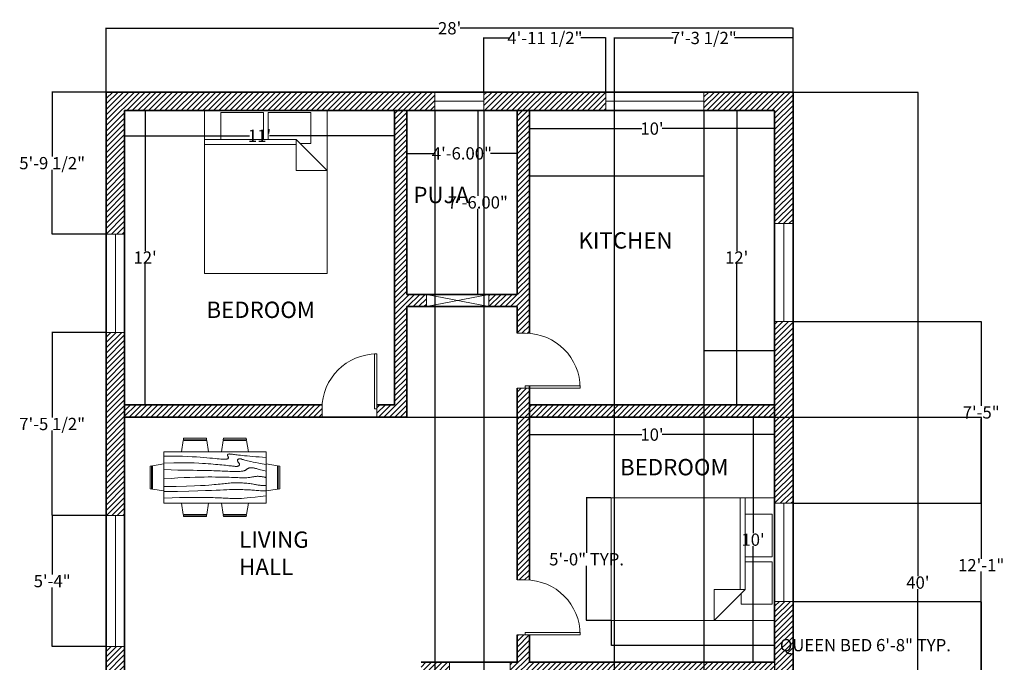
# Model space of a CAD drawing. Units: inches. Extents: x -20 to 887, y -143 to 410.
# Tile 5 of 5: x 401 to 883, y 96 to 410. Entities that reach past the tile are written whole.
import ezdxf

# ---------------------------------------------------------------- set-up
doc = ezdxf.new("R2010")
doc.units = ezdxf.units.IN
doc.header["$MEASUREMENT"] = 0
for name, color, linetype, lineweight in [('A-ANNO-DIMS', 2, 'Continuous', 18), ('A-AREA-IDEN', 7, 'Continuous', 25), ('A-DOOR', 3, 'Continuous', 18), ('A-FLOR-CASE', 9, 'Continuous', 25), ('A-FURN', 8, 'Continuous', 18), ('A-GLAZ', 4, 'Continuous', 18), ('A-WALL', 7, 'Continuous', 35), ('A-WALL-PATT', 8, 'Continuous', 13)]:
    doc.layers.add(name, color=color, linetype=linetype, lineweight=lineweight)
doc.styles.get("Standard").update_dxf_attribs({"font": 'arial.ttf'})
doc.dimstyles.get("Standard").update_dxf_attribs({"dimtxt": 6, "dimasz": 0.18, "dimexe": 0.18, "dimexo": 0.0625, "dimgap": 0.09, "dimtad": 0, "dimtih": 1, "dimtoh": 1, "dimzin": 0, "dimdsep": 46, "dimlunit": 3, "dimtxsty": 'Standard', "dimcen": 0.09, "dimadec": 0, "dimazin": 0, "dimtfac": 1, "dimtofl": 0, "dimtmove": 0, "dimatfit": 3, "dimfxl": 1, "dimtolj": 1, "dimtzin": 0, "dimarcsym": 0})

# ---------------------------------------------------------------- blocks, each defined once
blk = doc.blocks.new('Bed - Queen')
for p, q in [((0, -80.00003), (0, 0)), ((0, 0), (59.99999, 0)), ((59.99999, 0), (59.99999, -80.00003)), ((7.99999, -1.2), (28.79998, -1.2)), ((7.99999, -14.4), (7.99999, -1.2)), ((28.79998, -1.2), (28.79998, -14.4)), ((31.19999, -1.2), (51.99999, -1.2)), ((31.19999, -14.4), (31.19999, -1.2)), ((51.99999, -1.2), (51.99999, -16.4)), ((0, -14.4), (44.8, -14.4)), ((59.99999, -29.6), (44.8, -14.4)), ((44.8, -14.4), (44.8, -29.6)), ((44.8, -16.8), (0, -16.8)), ((51.99999, -16.4), (46.79936, -16.4)), ((44.8, -29.6), (59.99999, -29.6)), ((59.99999, -80.00003), (0, -80.00003))]:
    blk.add_line(p, q)
blk = doc.blocks.new('*U2')
for p, q in [((0, 0), (0, -6)), ((40, 0), (40, -6))]:
    blk.add_line(p, q)
blk.add_lwpolyline([(0, 0), (0, 40), (1.75, 40), (1.75, 0)], close=True)
blk.add_arc((0, 0), 40, 0, 90)
blk = doc.blocks.new('Dining Set - 36 x 72 in.')
for p, q in [((-22.2343, 26.00059), (-23.4847, 17.99762)), ((-22.2304, 26), (-5.7608, 26)), ((-22, 27.5), (-22.1562, 26.50042)), ((-5.8416, 26.5), (-22.1534, 26.5)), ((-22, 27.5), (-6, 27.5)), ((-5.8437, 26.49966), (-6, 27.5)), ((-4.5152, 17.99762), (-5.7655, 25.99926)), ((5.7657, 26.00059), (4.5153, 17.99762)), ((5.7696, 26), (22.2392, 26)), ((6, 27.5), (5.8438, 26.50042)), ((22.1584, 26.5), (5.8466, 26.5)), ((6, 27.5), (22, 27.5)), ((22.1563, 26.49966), (22, 27.5)), ((23.4848, 17.99762), (22.2345, 25.99926)), ((36, 18), (-36, 18)), ((-36, 18), (-36, -18)), ((36, -18), (36, 18)), ((-45.5, 8), (-44.5004, 8.15617)), ((-45.5, 8), (-45.5, -8)), ((-44.5, -8.15843), (-44.5, 8.15338)), ((-44.0006, 8.23428), (-35.9976, 9.48474)), ((-44, 8.23041), (-44, -8.23915)), ((44.0006, 8.23428), (35.9976, 9.48474)), ((44, 8.23041), (44, -8.23915)), ((44.5, -8.15843), (44.5, 8.15338)), ((45.5, 8), (44.5005, 8.15617)), ((45.5, 8), (45.5, -8)), ((-44.4997, -8.15631), (-45.5, -8)), ((-35.9976, -9.48476), (-43.9993, -8.2345)), ((35.9976, -9.48476), (43.9993, -8.2345)), ((44.4997, -8.15631), (45.5, -8)), ((-36, -18), (36, -18)), ((-22.2343, -26.0006), (-23.4847, -17.99762)), ((-4.5152, -17.99762), (-5.7655, -25.99928)), ((5.7657, -26.0006), (4.5153, -17.99762)), ((23.4848, -17.99762), (22.2345, -25.99928)), ((-22.2304, -26), (-5.7608, -26)), ((-22, -27.5), (-22.1562, -26.50044)), ((-5.8416, -26.5), (-22.1534, -26.5)), ((-22, -27.5), (-6, -27.5)), ((-5.8437, -26.49967), (-6, -27.5)), ((5.7696, -26), (22.2392, -26)), ((6, -27.5), (5.8438, -26.50044)), ((22.1584, -26.5), (5.8466, -26.5)), ((6, -27.5), (22, -27.5)), ((22.1563, -26.49967), (22, -27.5))]:
    blk.add_line(p, q)
for points in [[(-36, 15), (-31.1772, 14.97754), (-26.8079, 14.91406), (-22.8538, 14.81543), (-19.276, 14.6875), (-16.0362, 14.53613), (-13.0957, 14.36718), (-10.4159, 14.18652), (-7.9583, 14), (-5.6904, 13.81315), (-3.6035, 13.63021), (-1.6954, 13.45508), (0.0365, 13.29166), (1.5945, 13.14388), (2.9811, 13.01562), (4.1988, 12.9108), (5.25, 12.83333), (6.1393, 12.78613), (6.8802, 12.76823), (7.4883, 12.77767), (7.9792, 12.8125), (8.3685, 12.87077), (8.6719, 12.95052), (8.9049, 13.0498), (9.0833, 13.16666), (9.2205, 13.29899), (9.3216, 13.44401), (9.3895, 13.59879), (9.4271, 13.76041), (9.4373, 13.92594), (9.4232, 14.09245), (9.3875, 14.257), (9.3333, 14.41666), (9.2638, 14.56917), (9.1836, 14.71484), (9.0975, 14.85465), (9.0104, 14.98958), (8.9272, 15.1206), (8.8529, 15.2487), (8.7922, 15.37483), (8.75, 15.5), (8.7305, 15.62467), (8.7344, 15.74739), (8.7617, 15.86621), (8.8125, 15.97916), (8.8867, 16.08431), (8.9844, 16.17968), (9.1055, 16.26334), (9.25, 16.33333), (9.4189, 16.38802), (9.6172, 16.42708), (9.8506, 16.45052), (10.125, 16.45833), (10.4463, 16.45052), (10.8203, 16.42708), (11.2529, 16.38802), (11.75, 16.33333), (12.3184, 16.26318), (12.9694, 16.17838), (13.7151, 16.07991), (14.5677, 15.96875), (15.5395, 15.84586), (16.6426, 15.71224), (17.8893, 15.56884), (19.2917, 15.41666), (20.859, 15.25667), (22.5879, 15.08984), (24.4721, 14.91715), (26.5052, 14.73958), (28.6809, 14.5581), (30.9929, 14.3737), (33.4347, 14.18733), (36, 14)], [(-36, 10), (-28.9766, 10.14274), (-23.1725, 10.20442), (-18.4241, 10.19775), (-14.5677, 10.13541), (-11.4399, 10.03011), (-8.877, 9.89453), (-6.7154, 9.74137), (-4.7917, 9.58333), (-2.9698, 9.43082), (-1.2246, 9.28515), (0.4415, 9.14534), (2.026, 9.01041), (3.5266, 8.87939), (4.9408, 8.7513), (6.266, 8.62516), (7.5, 8.5), (8.6411, 8.37549), (9.6914, 8.2539), (10.6538, 8.13818), (11.5312, 8.03125), (12.3267, 7.93603), (13.043, 7.85547), (13.6831, 7.79248), (14.25, 7.75), (14.7471, 7.7303), (15.1797, 7.73307), (15.5537, 7.75732), (15.875, 7.80208), (16.1494, 7.86637), (16.3828, 7.94922), (16.5811, 8.04964), (16.75, 8.16666), (16.8944, 8.29915), (17.0143, 8.44531), (17.1089, 8.60319), (17.1771, 8.77083), (17.218, 8.94629), (17.2305, 9.1276), (17.2137, 9.31282), (17.1667, 9.5), (17.0895, 9.6875), (16.987, 9.875), (16.8649, 10.0625), (16.7292, 10.25), (16.5856, 10.4375), (16.4401, 10.625), (16.2985, 10.8125), (16.1667, 11), (16.05, 11.18733), (15.9518, 11.3737), (15.8752, 11.5581), (15.8229, 11.73958), (15.798, 11.91715), (15.8034, 12.08984), (15.842, 12.25667), (15.9167, 12.41666), (16.0295, 12.56836), (16.1784, 12.70833), (16.3605, 12.83268), (16.5729, 12.9375), (16.8127, 13.01888), (17.0768, 13.07291), (17.3625, 13.0957), (17.6667, 13.08333), (17.9894, 13.03312), (18.3418, 12.94726), (18.7382, 12.82918), (19.1927, 12.68229), (19.7195, 12.51001), (20.3327, 12.31575), (21.0465, 12.10294), (21.875, 11.875), (22.8357, 11.63354), (23.959, 11.37304), (25.2786, 11.08618), (26.8282, 10.76562), (28.6414, 10.40405), (30.752, 9.99414), (33.1936, 9.52856), (36, 9)], [(-36, 5.5), (-30.7157, 5.3348), (-26.069, 5.20963), (-21.9946, 5.11767), (-18.4271, 5.05208), (-15.3009, 5.00602), (-12.5508, 4.97265), (-10.1112, 4.94515), (-7.9167, 4.91666), (-5.909, 4.88167), (-4.0586, 4.83984), (-2.3429, 4.79215), (-0.7396, 4.73958), (0.7739, 4.6831), (2.22, 4.6237), (3.6213, 4.56233), (5, 4.5), (6.373, 4.43782), (7.7344, 4.3776), (9.0723, 4.32129), (10.375, 4.27083), (11.6309, 4.22819), (12.8281, 4.19531), (13.9551, 4.17415), (15, 4.16666), (15.954, 4.17448), (16.819, 4.19791), (17.6001, 4.23698), (18.3021, 4.29166), (18.9299, 4.36198), (19.4883, 4.44791), (19.9823, 4.54948), (20.4167, 4.66666), (20.7969, 4.79899), (21.1302, 4.94401), (21.4245, 5.09879), (21.6875, 5.26041), (21.9271, 5.42594), (22.1511, 5.59245), (22.3672, 5.757), (22.5834, 5.91666), (22.8065, 6.06868), (23.0404, 6.21093), (23.2879, 6.34147), (23.5521, 6.45833), (23.8358, 6.55957), (24.142, 6.64323), (24.4735, 6.70735), (24.8334, 6.75), (25.2235, 6.76969), (25.642, 6.76692), (26.0858, 6.74267), (26.5521, 6.69791), (27.0379, 6.63362), (27.5404, 6.55078), (28.0565, 6.45036), (28.5834, 6.33333), (29.1242, 6.19987), (29.7071, 6.04687), (30.3661, 5.87044), (31.1354, 5.66666), (32.0493, 5.43164), (33.142, 5.16146), (34.4475, 4.85221), (36, 4.5)], [(-36, -1), (-30.7915, -0.6591), (-26.0195, -0.38216), (-21.6519, -0.16284), (-17.6563, 0.00521), (-14.0005, 0.12833), (-10.6523, 0.21289), (-7.5796, 0.26522), (-4.75, 0.29166), (-2.134, 0.29793), (0.2878, 0.28711), (2.5317, 0.26163), (4.6146, 0.22396), (6.5529, 0.17651), (8.3633, 0.12174), (10.0623, 0.06209), (11.6667, 0), (13.1899, -0.06201), (14.6341, -0.1211), (15.9982, -0.17432), (17.2813, -0.21875), (18.4823, -0.25147), (19.6003, -0.26953), (20.6343, -0.27002), (21.5834, -0.25), (22.4481, -0.20768), (23.2357, -0.14584), (23.9549, -0.06836), (24.6146, 0.02083), (25.2235, 0.11784), (25.7904, 0.21875), (26.3241, 0.31966), (26.8334, 0.41666), (27.3265, 0.50618), (27.8099, 0.58593), (28.2894, 0.65397), (28.7709, 0.70833), (29.2601, 0.74707), (29.763, 0.76823), (30.2855, 0.76985), (30.8334, 0.75), (31.4088, 0.70784), (31.9994, 0.64713), (32.589, 0.57275), (33.1615, 0.48958), (33.7008, 0.4025), (34.1908, 0.3164), (34.6153, 0.23616), (34.9584, 0.16666), (35.2099, 0.11165), (35.3848, 0.07031), (35.504, 0.04069), (35.5886, 0.02083), (35.6594, 0.00879), (35.7377, 0.0026), (35.8442, 0.00032), (36, 0)], [(-36, -6.5), (-27.1843, -6.31267), (-20.084, -6.1263), (-14.469, -5.9419), (-10.1094, -5.76042), (-6.7752, -5.58285), (-4.2363, -5.41016), (-2.2629, -5.24333), (-0.625, -5.08334), (0.8708, -4.93099), (2.2715, -4.78646), (3.5872, -4.64974), (4.8281, -4.52084), (6.0046, -4.39974), (7.127, -4.28646), (8.2053, -4.18099), (9.25, -4.08334), (10.2705, -3.99382), (11.2734, -3.91407), (12.2647, -3.84603), (13.25, -3.79167), (14.2354, -3.75293), (15.2266, -3.73177), (16.2295, -3.73015), (17.25, -3.75), (18.2912, -3.79248), (19.3451, -3.85547), (20.4009, -3.93604), (21.4479, -4.03125), (22.4754, -4.13819), (23.4727, -4.25391), (24.4289, -4.37549), (25.3334, -4.5), (26.1785, -4.62492), (26.9694, -4.74935), (27.7145, -4.87281), (28.4219, -4.99479), (29.1, -5.11483), (29.7572, -5.23242), (30.4016, -5.34709), (31.0417, -5.45834), (31.6837, -5.56437), (32.3262, -5.65821), (32.9658, -5.73153), (33.599, -5.77604), (34.2224, -5.78345), (34.8327, -5.74545), (35.4264, -5.65373), (36, -5.5)], [(-36, -10), (-26.4022, -9.81299), (-18.4675, -9.62891), (-11.9839, -9.45069), (-6.7396, -9.28125), (-2.5226, -9.12354), (0.8789, -8.98047), (3.6769, -8.85498), (6.0833, -8.75), (8.2767, -8.66765), (10.3021, -8.60677), (12.1712, -8.56543), (13.8958, -8.54167), (15.4876, -8.53353), (16.9583, -8.53907), (18.3197, -8.55632), (19.5834, -8.58334), (20.7616, -8.61841), (21.8685, -8.66081), (22.9188, -8.71004), (23.9271, -8.76563), (24.9081, -8.82707), (25.8763, -8.89388), (26.8465, -8.96558), (27.8334, -9.04167), (28.8474, -9.12118), (29.8828, -9.20117), (30.93, -9.27824), (31.9792, -9.34896), (33.0205, -9.40991), (34.0443, -9.45768), (35.0407, -9.48885), (36, -9.5)], [(-36, -14.5), (-30.0881, -14.33513), (-25.0332, -14.21224), (-20.7312, -14.12647), (-17.0781, -14.07292), (-13.97, -14.04671), (-11.3027, -14.04297), (-8.9724, -14.05681), (-6.875, -14.08334), (-4.9224, -14.11833), (-3.0905, -14.16016), (-1.3709, -14.20785), (0.2448, -14.26042), (1.7647, -14.3169), (3.1973, -14.3763), (4.5507, -14.43767), (5.8333, -14.5), (7.0554, -14.5621), (8.235, -14.62175), (9.3922, -14.67652), (10.5469, -14.72396), (11.7192, -14.76164), (12.929, -14.78711), (14.1965, -14.79794), (15.5417, -14.79167), (16.9933, -14.76424), (18.6152, -14.70508), (20.4804, -14.60197), (22.6615, -14.44271), (25.2312, -14.21509), (28.2624, -13.9069), (31.8277, -13.50594), (36, -13)]]:
    blk.add_lwpolyline(points)
blk = doc.blocks.new('*D25')
at = {"layer": 'A-ANNO-DIMS', "color": 0, "lineweight": -2, "transparency": 16777216}
for p, q in [((443.33, 374.98), (443.33, 406.3)), ((443.51, 406.12), (606.1, 406.12)), ((779.15, 406.12), (616.56, 406.12)), ((779.33, 374.98), (779.33, 406.3))]:
    blk.add_line(p, q, dxfattribs=at)
at = {"layer": 'A-ANNO-DIMS', "color": 0, "transparency": 16777216}
for points in [[(443.51, 406.15), (443.51, 406.09), (443.33, 406.12)], [(779.15, 406.15), (779.15, 406.09), (779.33, 406.12)]]:
    blk.add_solid(points, dxfattribs=at)
at = {"layer": 'Defpoints', "color": 0, "transparency": 16777216}
for p in [(779.33, 406.12), (443.33, 374.92), (779.33, 374.92)]:
    blk.add_point(p, dxfattribs=at)
at = {"layer": 'A-ANNO-DIMS', "color": 0, "transparency": 16777216, "insert": (611.33, 406.12), "char_height": 6, "attachment_point": 5}
blk.add_mtext("\\A1;28'", dxfattribs=at)
blk = doc.blocks.new('*D26')
at = {"layer": 'A-ANNO-DIMS', "color": 0, "lineweight": -2, "transparency": 16777216}
for p, q in [((779.39, 374.92), (840.59, 374.92)), ((840.41, 374.74), (840.41, 138.07)), ((840.41, -104.9), (840.41, 131.76)), ((779.39, -105.08), (840.59, -105.08))]:
    blk.add_line(p, q, dxfattribs=at)
at = {"layer": 'A-ANNO-DIMS', "color": 0, "transparency": 16777216}
for points in [[(840.38, 374.74), (840.44, 374.74), (840.41, 374.92)], [(840.38, -104.9), (840.44, -104.9), (840.41, -105.08)]]:
    blk.add_solid(points, dxfattribs=at)
at = {"layer": 'Defpoints', "color": 0, "transparency": 16777216}
for p in [(779.33, 374.92), (779.33, -105.08), (840.41, -105.08)]:
    blk.add_point(p, dxfattribs=at)
at = {"layer": 'A-ANNO-DIMS', "color": 0, "transparency": 16777216, "insert": (840.41, 134.92), "char_height": 6, "attachment_point": 5}
blk.add_mtext("\\A1;40'", dxfattribs=at)
blk = doc.blocks.new('*D34')
at = {"layer": 'A-ANNO-DIMS', "color": 0, "lineweight": -2, "transparency": 16777216}
for p, q in [((770.27, 215.92), (759.59, 215.92)), ((759.77, 215.74), (759.77, 159.07)), ((759.77, 96.1), (759.77, 152.76)), ((770.27, 95.92), (759.59, 95.92))]:
    blk.add_line(p, q, dxfattribs=at)
at = {"layer": 'A-ANNO-DIMS', "color": 0, "transparency": 16777216}
for points in [[(759.74, 215.74), (759.8, 215.74), (759.77, 215.92)], [(759.74, 96.1), (759.8, 96.1), (759.77, 95.92)]]:
    blk.add_solid(points, dxfattribs=at)
at = {"layer": 'Defpoints', "color": 0, "transparency": 16777216}
for p in [(770.33, 215.92), (759.77, 95.92), (770.33, 95.92)]:
    blk.add_point(p, dxfattribs=at)
at = {"layer": 'A-ANNO-DIMS', "color": 0, "transparency": 16777216, "insert": (759.77, 155.92), "char_height": 6, "attachment_point": 5}
blk.add_mtext("\\A1;10'", dxfattribs=at)
blk = doc.blocks.new('*D35')
at = {"layer": 'A-ANNO-DIMS', "color": 0, "lineweight": -2, "transparency": 16777216}
for p, q in [((650.33, 215.86), (650.33, 207.13)), ((770.33, 215.86), (770.33, 207.13)), ((650.51, 207.31), (705.43, 207.31)), ((770.15, 207.31), (715.23, 207.31))]:
    blk.add_line(p, q, dxfattribs=at)
at = {"layer": 'A-ANNO-DIMS', "color": 0, "transparency": 16777216}
for points in [[(650.51, 207.34), (650.51, 207.28), (650.33, 207.31)], [(770.15, 207.34), (770.15, 207.28), (770.33, 207.31)]]:
    blk.add_solid(points, dxfattribs=at)
at = {"layer": 'Defpoints', "color": 0, "transparency": 16777216}
for p in [(650.33, 215.92), (770.33, 215.92), (770.33, 207.31)]:
    blk.add_point(p, dxfattribs=at)
at = {"layer": 'A-ANNO-DIMS', "color": 0, "transparency": 16777216, "insert": (710.33, 207.31), "char_height": 6, "attachment_point": 5}
blk.add_mtext("\\A1;10'", dxfattribs=at)
blk = doc.blocks.new('*D36')
at = {"layer": 'A-ANNO-DIMS', "color": 0, "lineweight": -2, "transparency": 16777216}
for p, q in [((644.27, 365.92), (624.93, 365.92)), ((625.11, 365.74), (625.11, 324.07)), ((625.11, 276.1), (625.11, 317.76)), ((644.27, 275.92), (624.93, 275.92))]:
    blk.add_line(p, q, dxfattribs=at)
at = {"layer": 'A-ANNO-DIMS', "color": 0, "transparency": 16777216}
for points in [[(625.08, 365.74), (625.14, 365.74), (625.11, 365.92)], [(625.08, 276.1), (625.14, 276.1), (625.11, 275.92)]]:
    blk.add_solid(points, dxfattribs=at)
at = {"layer": 'Defpoints', "color": 0, "transparency": 16777216}
for p in [(644.33, 365.92), (625.11, 275.92), (644.33, 275.92)]:
    blk.add_point(p, dxfattribs=at)
at = {"layer": 'A-ANNO-DIMS', "color": 0, "transparency": 16777216, "insert": (625.11, 320.92), "char_height": 6, "attachment_point": 5}
blk.add_mtext('\\A1;7\'-6.00"', dxfattribs=at)
blk = doc.blocks.new('*D37')
at = {"layer": 'A-ANNO-DIMS', "color": 0, "lineweight": -2, "transparency": 16777216}
for p, q in [((590.33, 365.86), (590.33, 344.72)), ((644.33, 365.86), (644.33, 344.72)), ((590.51, 344.9), (603.32, 344.9)), ((644.15, 344.9), (631.34, 344.9))]:
    blk.add_line(p, q, dxfattribs=at)
at = {"layer": 'A-ANNO-DIMS', "color": 0, "transparency": 16777216}
for points in [[(590.51, 344.93), (590.51, 344.87), (590.33, 344.9)], [(644.15, 344.93), (644.15, 344.87), (644.33, 344.9)]]:
    blk.add_solid(points, dxfattribs=at)
at = {"layer": 'Defpoints', "color": 0, "transparency": 16777216}
for p in [(590.33, 365.92), (644.33, 365.92), (644.33, 344.9)]:
    blk.add_point(p, dxfattribs=at)
at = {"layer": 'A-ANNO-DIMS', "color": 0, "transparency": 16777216, "insert": (617.33, 344.9), "char_height": 6, "attachment_point": 5}
blk.add_mtext('\\A1;4\'-6.00"', dxfattribs=at)
blk = doc.blocks.new('*D38')
at = {"layer": 'A-ANNO-DIMS', "color": 0, "lineweight": -2, "transparency": 16777216}
for p, q in [((650.33, 365.86), (650.33, 356.85)), ((770.33, 365.86), (770.33, 356.85)), ((650.51, 357.03), (705.43, 357.03)), ((770.15, 357.03), (715.23, 357.03))]:
    blk.add_line(p, q, dxfattribs=at)
at = {"layer": 'A-ANNO-DIMS', "color": 0, "transparency": 16777216}
for points in [[(650.51, 357.06), (650.51, 357), (650.33, 357.03)], [(770.15, 357.06), (770.15, 357), (770.33, 357.03)]]:
    blk.add_solid(points, dxfattribs=at)
at = {"layer": 'Defpoints', "color": 0, "transparency": 16777216}
for p in [(650.33, 365.92), (770.33, 365.92), (770.33, 357.03)]:
    blk.add_point(p, dxfattribs=at)
at = {"layer": 'A-ANNO-DIMS', "color": 0, "transparency": 16777216, "insert": (710.33, 357.03), "char_height": 6, "attachment_point": 5}
blk.add_mtext("\\A1;10'", dxfattribs=at)
blk = doc.blocks.new('*D39')
at = {"layer": 'A-ANNO-DIMS', "color": 0, "lineweight": -2, "transparency": 16777216}
for p, q in [((770.27, 365.92), (751.58, 365.92)), ((751.76, 365.74), (751.76, 297.02)), ((751.76, 222.1), (751.76, 290.82)), ((770.27, 221.92), (751.58, 221.92))]:
    blk.add_line(p, q, dxfattribs=at)
at = {"layer": 'A-ANNO-DIMS', "color": 0, "transparency": 16777216}
for points in [[(751.73, 365.74), (751.79, 365.74), (751.76, 365.92)], [(751.73, 222.1), (751.79, 222.1), (751.76, 221.92)]]:
    blk.add_solid(points, dxfattribs=at)
at = {"layer": 'Defpoints', "color": 0, "transparency": 16777216}
for p in [(770.33, 365.92), (751.76, 221.92), (770.33, 221.92)]:
    blk.add_point(p, dxfattribs=at)
at = {"layer": 'A-ANNO-DIMS', "color": 0, "transparency": 16777216, "insert": (751.76, 293.92), "char_height": 6, "attachment_point": 5}
blk.add_mtext("\\A1;12'", dxfattribs=at)
blk = doc.blocks.new('*D40')
at = {"layer": 'A-ANNO-DIMS', "color": 0, "lineweight": -2, "transparency": 16777216}
for p, q in [((452.39, 365.92), (462.53, 365.92)), ((462.35, 365.74), (462.35, 297.02)), ((462.35, 222.1), (462.35, 290.82)), ((452.39, 221.92), (462.53, 221.92))]:
    blk.add_line(p, q, dxfattribs=at)
at = {"layer": 'A-ANNO-DIMS', "color": 0, "transparency": 16777216}
for points in [[(462.32, 365.74), (462.38, 365.74), (462.35, 365.92)], [(462.32, 222.1), (462.38, 222.1), (462.35, 221.92)]]:
    blk.add_solid(points, dxfattribs=at)
at = {"layer": 'Defpoints', "color": 0, "transparency": 16777216}
for p in [(452.33, 365.92), (462.35, 365.92), (452.33, 221.92)]:
    blk.add_point(p, dxfattribs=at)
at = {"layer": 'A-ANNO-DIMS', "color": 0, "transparency": 16777216, "insert": (462.35, 293.92), "char_height": 6, "attachment_point": 5}
blk.add_mtext("\\A1;12'", dxfattribs=at)
blk = doc.blocks.new('*D41')
at = {"layer": 'A-ANNO-DIMS', "color": 0, "lineweight": -2, "transparency": 16777216}
for p, q in [((452.33, 365.86), (452.33, 353.34)), ((584.33, 365.86), (584.33, 353.34)), ((452.51, 353.52), (513.43, 353.52)), ((584.15, 353.52), (523.23, 353.52))]:
    blk.add_line(p, q, dxfattribs=at)
at = {"layer": 'A-ANNO-DIMS', "color": 0, "transparency": 16777216}
for points in [[(452.51, 353.55), (452.51, 353.49), (452.33, 353.52)], [(584.15, 353.55), (584.15, 353.49), (584.33, 353.52)]]:
    blk.add_solid(points, dxfattribs=at)
at = {"layer": 'Defpoints', "color": 0, "transparency": 16777216}
for p in [(452.33, 365.92), (584.33, 365.92), (584.33, 353.52)]:
    blk.add_point(p, dxfattribs=at)
at = {"layer": 'A-ANNO-DIMS', "color": 0, "transparency": 16777216, "insert": (518.33, 353.52), "char_height": 6, "attachment_point": 5}
blk.add_mtext("\\A1;11'", dxfattribs=at)
blk = doc.blocks.new('WIN-48IN-9IN-WALL')
for p, q in [((9, 48), (0, 48)), ((4.5, 0), (4.5, 48)), ((9, 0), (0, 0))]:
    blk.add_line(p, q)
blk = doc.blocks.new('*D45')
at = {"layer": 'A-ANNO-DIMS', "color": 0, "lineweight": -2, "transparency": 16777216}
for p, q in [((690.33, 116.26), (690.33, 104.14)), ((770.33, 116.26), (770.33, 104.14)), ((690.51, 104.32), (770.15, 104.32)), ((770.33, 104.32), (770.51, 104.32))]:
    blk.add_line(p, q, dxfattribs=at)
at = {"layer": 'A-ANNO-DIMS', "color": 0, "transparency": 16777216}
for points in [[(690.51, 104.35), (690.51, 104.29), (690.33, 104.32)], [(770.15, 104.35), (770.15, 104.29), (770.33, 104.32)]]:
    blk.add_solid(points, dxfattribs=at)
at = {"layer": 'Defpoints', "color": 0, "transparency": 16777216}
for p in [(690.33, 116.32), (770.33, 116.32), (770.33, 104.32)]:
    blk.add_point(p, dxfattribs=at)
at = {"layer": 'A-ANNO-DIMS', "color": 0, "transparency": 16777216, "insert": (814.73, 104.32), "char_height": 6, "attachment_point": 5}
blk.add_mtext('\\A1;QUEEN BED 6\'-8" TYP.', dxfattribs=at)
blk = doc.blocks.new('*D46')
at = {"layer": 'A-ANNO-DIMS', "color": 0, "lineweight": -2, "transparency": 16777216}
for p, q in [((690.27, 176.32), (678.15, 176.32)), ((678.33, 176.14), (678.33, 149.47)), ((678.33, 116.5), (678.33, 143.17)), ((690.27, 116.32), (678.15, 116.32))]:
    blk.add_line(p, q, dxfattribs=at)
at = {"layer": 'A-ANNO-DIMS', "color": 0, "transparency": 16777216}
for points in [[(678.3, 176.14), (678.36, 176.14), (678.33, 176.32)], [(678.3, 116.5), (678.36, 116.5), (678.33, 116.32)]]:
    blk.add_solid(points, dxfattribs=at)
at = {"layer": 'Defpoints', "color": 0, "transparency": 16777216}
for p in [(690.33, 176.32), (678.33, 116.32), (690.33, 116.32)]:
    blk.add_point(p, dxfattribs=at)
at = {"layer": 'A-ANNO-DIMS', "color": 0, "transparency": 16777216, "insert": (678.33, 146.32), "char_height": 6, "attachment_point": 5}
blk.add_mtext('\\A1;5\'-0" TYP.', dxfattribs=at)
blk = doc.blocks.new('*D75')
at = {"layer": 'A-ANNO-DIMS', "color": 0, "lineweight": -2, "transparency": 16777216}
for p, q in [((692.01, -57.02), (692.01, 401.55)), ((692.19, 401.37), (720.64, 401.37)), ((779.15, 401.37), (750.7, 401.37)), ((779.33, -57.02), (779.33, 401.55))]:
    blk.add_line(p, q, dxfattribs=at)
at = {"layer": 'A-ANNO-DIMS', "color": 0, "transparency": 16777216}
for points in [[(692.19, 401.4), (692.19, 401.34), (692.01, 401.37)], [(779.15, 401.4), (779.15, 401.34), (779.33, 401.37)]]:
    blk.add_solid(points, dxfattribs=at)
at = {"layer": 'Defpoints', "color": 0, "transparency": 16777216}
for p in [(779.33, 401.37), (692.01, -57.08), (779.33, -57.08)]:
    blk.add_point(p, dxfattribs=at)
at = {"layer": 'A-ANNO-DIMS', "color": 0, "transparency": 16777216, "insert": (735.67, 401.37), "char_height": 6, "attachment_point": 5}
blk.add_mtext('\\A1;7\'-3 1/2"', dxfattribs=at)
blk = doc.blocks.new('*D77')
at = {"layer": 'A-ANNO-DIMS', "color": 0, "lineweight": -2, "transparency": 16777216}
for p, q in [((779.39, 125.72), (871.56, 125.72)), ((871.38, 125.54), (871.38, 85.75)), ((871.38, 39.75), (871.38, 79.55)), ((779.39, 39.57), (871.56, 39.57))]:
    blk.add_line(p, q, dxfattribs=at)
at = {"layer": 'A-ANNO-DIMS', "color": 0, "transparency": 16777216}
for points in [[(871.35, 125.54), (871.41, 125.54), (871.38, 125.72)], [(871.35, 39.75), (871.41, 39.75), (871.38, 39.57)]]:
    blk.add_solid(points, dxfattribs=at)
at = {"layer": 'Defpoints', "color": 0, "transparency": 16777216}
for p in [(779.33, 125.72), (871.38, 125.72), (779.33, 39.57)]:
    blk.add_point(p, dxfattribs=at)
at = {"layer": 'A-ANNO-DIMS', "color": 0, "transparency": 16777216, "insert": (871.38, 82.65), "char_height": 6, "attachment_point": 5}
blk.add_mtext('\\A1;7\'-2"', dxfattribs=at)
blk = doc.blocks.new('*D78')
at = {"layer": 'A-ANNO-DIMS', "color": 0, "lineweight": -2, "transparency": 16777216}
for p, q in [((779.39, 262.64), (871.56, 262.64)), ((871.38, 262.46), (871.38, 221.32)), ((871.38, 173.9), (871.38, 215.04)), ((779.39, 173.72), (871.56, 173.72))]:
    blk.add_line(p, q, dxfattribs=at)
at = {"layer": 'A-ANNO-DIMS', "color": 0, "transparency": 16777216}
for points in [[(871.35, 262.46), (871.41, 262.46), (871.38, 262.64)], [(871.35, 173.9), (871.41, 173.9), (871.38, 173.72)]]:
    blk.add_solid(points, dxfattribs=at)
at = {"layer": 'Defpoints', "color": 0, "transparency": 16777216}
for p in [(779.33, 262.64), (871.38, 262.64), (779.33, 173.72)]:
    blk.add_point(p, dxfattribs=at)
at = {"layer": 'A-ANNO-DIMS', "color": 0, "transparency": 16777216, "insert": (871.38, 218.18), "char_height": 6, "attachment_point": 5}
blk.add_mtext('\\A1;7\'-5"', dxfattribs=at)
blk = doc.blocks.new('*D79')
at = {"layer": 'A-ANNO-DIMS', "color": 0, "lineweight": -2, "transparency": 16777216}
for p, q in [((735.77, 365.86), (735.77, -134.33)), ((770.33, 365.86), (770.33, -134.33)), ((735.95, -134.15), (770.15, -134.15)), ((770.33, -134.15), (770.51, -134.15))]:
    blk.add_line(p, q, dxfattribs=at)
at = {"layer": 'A-ANNO-DIMS', "color": 0, "transparency": 16777216}
for points in [[(735.95, -134.12), (735.95, -134.18), (735.77, -134.15)], [(770.15, -134.12), (770.15, -134.18), (770.33, -134.15)]]:
    blk.add_solid(points, dxfattribs=at)
at = {"layer": 'Defpoints', "color": 0, "transparency": 16777216}
for p in [(735.77, 365.92), (770.33, 365.92), (770.33, -134.15)]:
    blk.add_point(p, dxfattribs=at)
at = {"layer": 'A-ANNO-DIMS', "color": 0, "transparency": 16777216, "insert": (787.95, -134.15), "char_height": 6, "attachment_point": 5}
blk.add_mtext('\\A1;2\'-10 1/2"', dxfattribs=at)
blk = doc.blocks.new('*D80')
at = {"layer": 'A-ANNO-DIMS', "color": 0, "lineweight": -2, "transparency": 16777216}
for p, q in [((628.12, 374.98), (628.12, 401.55)), ((628.3, 401.37), (640.44, 401.37)), ((687.59, 401.37), (675.45, 401.37)), ((687.77, 374.98), (687.77, 401.55))]:
    blk.add_line(p, q, dxfattribs=at)
at = {"layer": 'A-ANNO-DIMS', "color": 0, "transparency": 16777216}
for points in [[(628.3, 401.4), (628.3, 401.34), (628.12, 401.37)], [(687.59, 401.4), (687.59, 401.34), (687.77, 401.37)]]:
    blk.add_solid(points, dxfattribs=at)
at = {"layer": 'Defpoints', "color": 0, "transparency": 16777216}
for p in [(687.77, 401.37), (628.12, 374.92), (687.77, 374.92)]:
    blk.add_point(p, dxfattribs=at)
at = {"layer": 'A-ANNO-DIMS', "color": 0, "transparency": 16777216, "insert": (657.95, 401.37), "char_height": 6, "attachment_point": 5}
blk.add_mtext('\\A1;4\'-11 1/2"', dxfattribs=at)
blk = doc.blocks.new('*D81')
at = {"layer": 'A-ANNO-DIMS', "color": 0, "lineweight": -2, "transparency": 16777216}
for p, q in [((604.12, 365.86), (604.12, -134.33)), ((628.12, 365.86), (628.12, -134.33)), ((604.3, -134.15), (608.01, -134.15)), ((627.94, -134.15), (624.24, -134.15))]:
    blk.add_line(p, q, dxfattribs=at)
at = {"layer": 'A-ANNO-DIMS', "color": 0, "transparency": 16777216}
for points in [[(604.3, -134.12), (604.3, -134.18), (604.12, -134.15)], [(627.94, -134.12), (627.94, -134.18), (628.12, -134.15)]]:
    blk.add_solid(points, dxfattribs=at)
at = {"layer": 'Defpoints', "color": 0, "transparency": 16777216}
for p in [(604.12, 365.92), (628.12, 365.92), (628.12, -134.15)]:
    blk.add_point(p, dxfattribs=at)
at = {"layer": 'A-ANNO-DIMS', "color": 0, "transparency": 16777216, "insert": (616.12, -134.15), "char_height": 6, "attachment_point": 5}
blk.add_mtext('\\A1;2\'-0"', dxfattribs=at)
blk = doc.blocks.new('*D82')
at = {"layer": 'A-ANNO-DIMS', "color": 0, "lineweight": -2, "transparency": 16777216}
for p, q in [((443.27, 374.92), (416.7, 374.92)), ((416.88, 374.74), (416.88, 343.33)), ((416.88, 305.53), (416.88, 336.94)), ((443.27, 305.35), (416.7, 305.35))]:
    blk.add_line(p, q, dxfattribs=at)
at = {"layer": 'A-ANNO-DIMS', "color": 0, "transparency": 16777216}
for points in [[(416.85, 374.74), (416.91, 374.74), (416.88, 374.92)], [(416.85, 305.53), (416.91, 305.53), (416.88, 305.35)]]:
    blk.add_solid(points, dxfattribs=at)
at = {"layer": 'Defpoints', "color": 0, "transparency": 16777216}
for p in [(416.88, 374.92), (443.33, 374.92), (443.33, 305.35)]:
    blk.add_point(p, dxfattribs=at)
at = {"layer": 'A-ANNO-DIMS', "color": 0, "transparency": 16777216, "insert": (416.88, 340.13), "char_height": 6, "attachment_point": 5}
blk.add_mtext('\\A1;5\'-9 1/2"', dxfattribs=at)
blk = doc.blocks.new('*D83')
at = {"layer": 'A-ANNO-DIMS', "color": 0, "lineweight": -2, "transparency": 16777216}
for p, q in [((443.27, 257.35), (416.7, 257.35)), ((416.88, 257.17), (416.88, 215.71)), ((416.88, 167.86), (416.88, 209.32)), ((443.27, 167.68), (416.7, 167.68))]:
    blk.add_line(p, q, dxfattribs=at)
at = {"layer": 'A-ANNO-DIMS', "color": 0, "transparency": 16777216}
for points in [[(416.85, 257.17), (416.91, 257.17), (416.88, 257.35)], [(416.85, 167.86), (416.91, 167.86), (416.88, 167.68)]]:
    blk.add_solid(points, dxfattribs=at)
at = {"layer": 'Defpoints', "color": 0, "transparency": 16777216}
for p in [(416.88, 257.35), (443.33, 257.35), (443.33, 167.68)]:
    blk.add_point(p, dxfattribs=at)
at = {"layer": 'A-ANNO-DIMS', "color": 0, "transparency": 16777216, "insert": (416.88, 212.52), "char_height": 6, "attachment_point": 5}
blk.add_mtext('\\A1;7\'-5 1/2"', dxfattribs=at)
blk = doc.blocks.new('*D84')
at = {"layer": 'A-ANNO-DIMS', "color": 0, "lineweight": -2, "transparency": 16777216}
for p, q in [((443.27, 167.68), (416.7, 167.68)), ((416.88, 167.5), (416.88, 138.81)), ((416.88, 103.83), (416.88, 132.53)), ((443.27, 103.65), (416.7, 103.65))]:
    blk.add_line(p, q, dxfattribs=at)
at = {"layer": 'A-ANNO-DIMS', "color": 0, "transparency": 16777216}
for points in [[(416.85, 167.5), (416.91, 167.5), (416.88, 167.68)], [(416.85, 103.83), (416.91, 103.83), (416.88, 103.65)]]:
    blk.add_solid(points, dxfattribs=at)
at = {"layer": 'Defpoints', "color": 0, "transparency": 16777216}
for p in [(416.88, 167.68), (443.33, 167.68), (443.33, 103.65)]:
    blk.add_point(p, dxfattribs=at)
at = {"layer": 'A-ANNO-DIMS', "color": 0, "transparency": 16777216, "insert": (416.88, 135.67), "char_height": 6, "attachment_point": 5}
blk.add_mtext('\\A1;5\'-4"', dxfattribs=at)
blk = doc.blocks.new('*D85')
at = {"layer": 'A-ANNO-DIMS', "color": 0, "lineweight": -2, "transparency": 16777216}
for p, q in [((452.39, 215.92), (871.56, 215.92)), ((871.38, 215.74), (871.38, 146.52)), ((871.38, 71.1), (871.38, 140.32)), ((452.39, 70.92), (871.56, 70.92))]:
    blk.add_line(p, q, dxfattribs=at)
at = {"layer": 'A-ANNO-DIMS', "color": 0, "transparency": 16777216}
for points in [[(871.35, 215.74), (871.41, 215.74), (871.38, 215.92)], [(871.35, 71.1), (871.41, 71.1), (871.38, 70.92)]]:
    blk.add_solid(points, dxfattribs=at)
at = {"layer": 'Defpoints', "color": 0, "transparency": 16777216}
for p in [(452.33, 215.92), (452.33, 70.92), (871.38, 70.92)]:
    blk.add_point(p, dxfattribs=at)
at = {"layer": 'A-ANNO-DIMS', "color": 0, "transparency": 16777216, "insert": (871.38, 143.42), "char_height": 6, "attachment_point": 5}
blk.add_mtext('\\A1;12\'-1"', dxfattribs=at)

msp = doc.modelspace()

# ---------------------------------------------------------------- hatches: boundary and pattern name
at = {"layer": 'A-WALL-PATT'}
h = msp.add_hatch(dxfattribs=at)
h.set_pattern_fill('ANSI31', color=256, scale=15)
h.paths.add_polyline_path([(452.328, 365.918), (491.435, 365.918), (491.435, 366.063), (551.435, 366.063), (604.122, 366.028), (604.122, 374.918), (443.328, 374.918), (443.328, 305.35), (452.328, 305.35)])
h = msp.add_hatch(dxfattribs=at)
h.set_pattern_fill('ANSI31', color=256, scale=15)
h.paths.add_polyline_path([(687.77, 374.918), (628.122, 374.918), (628.122, 365.918), (687.77, 365.918)])
h = msp.add_hatch(dxfattribs=at)
h.set_pattern_fill('ANSI31', color=256, scale=15)
h.paths.add_polyline_path([(779.328, 374.918), (735.77, 374.918), (735.77, 365.918), (770.328, 365.918), (770.328, 310.637), (779.328, 310.637)])
h = msp.add_hatch(dxfattribs=at)
h.set_pattern_fill('ANSI31', color=256, scale=15)
h.paths.add_polyline_path([(590.328, 269.918), (599.942, 269.918), (599.942, 275.918), (590.328, 275.918), (590.328, 365.918), (584.328, 365.918), (584.328, 221.918), (575.752, 221.918), (575.752, 219.946), (575.752, 215.918), (590.328, 215.918)])
h = msp.add_hatch(dxfattribs=at)
h.set_pattern_fill('ANSI31', color=256, scale=15)
h.paths.add_polyline_path([(650.328, 365.918), (644.328, 365.918), (644.328, 275.918), (630.491, 275.918), (630.491, 269.918), (644.328, 269.918), (644.328, 256.868), (648.356, 256.868, -0.0183735), (650.328, 256.796)])
h = msp.add_hatch(dxfattribs=at)
h.set_pattern_fill('ANSI31', color=256, scale=15)
h.paths.add_polyline_path([(779.328, 262.637), (770.328, 262.637), (770.328, 173.723), (779.328, 173.723)])
h.paths.add_polyline_path([(770.328, 221.918), (650.328, 221.918), (650.328, 215.918), (770.328, 215.918)])
h = msp.add_hatch(dxfattribs=at)
h.set_pattern_fill('ANSI31', color=256, scale=15)
h.paths.add_polyline_path([(452.328, 257.35), (443.328, 257.35), (443.328, 167.684), (452.328, 167.684)])
h = msp.add_hatch(dxfattribs=at)
h.set_pattern_fill('ANSI31', color=256, scale=15)
h.paths.add_polyline_path([(650.328, 230.013), (648.356, 230.013), (644.328, 230.013), (644.328, 136.208), (648.356, 136.208, -0.0183735), (650.328, 136.135)])
h = msp.add_hatch(dxfattribs=at)
h.set_pattern_fill('ANSI31', color=256, scale=15)
h.paths.add_polyline_path([(548.897, 219.946, -0.0183735), (548.969, 221.918), (452.328, 221.918), (452.328, 215.918), (548.897, 215.918)])
h = msp.add_hatch(dxfattribs=at)
h.set_pattern_fill('ANSI31', color=256, scale=15)
h.paths.add_polyline_path([(779.328, 125.723), (770.328, 125.723), (770.328, 116.321), (770.328, 95.918), (650.328, 95.918), (650.328, 109.352), (648.356, 109.352), (644.328, 109.352), (644.328, 95.918), (640.97, 95.918), (640.97, 91.453, -0.0129025), (640.93, 89.918), (770.328, 89.918), (770.328, 39.573), (779.328, 39.573)])
h.paths.add_polyline_path([(779.328, -8.427), (770.328, -8.427), (770.328, -48.082), (692.012, -48.082), (692.012, -57.082), (779.328, -57.082)])
h.paths.add_polyline_path([(644.012, -48.082), (587.007, -48.082), (587.007, -57.082), (644.012, -57.082)])
h.paths.add_polyline_path([(603.328, 89.918), (611.206, 89.918), (611.206, 91.453), (611.206, 95.918), (597.328, 95.918), (597.328, 41.918), (565.317, 41.918), (565.317, 39.309, -0.049098), (564.984, 35.918), (597.328, 35.918), (597.328, -48.082), (603.328, -48.082)])
h.paths.add_polyline_path([(545.328, -57.082), (554.942, -57.082), (554.942, -48.082), (536.328, -48.082), (536.328, -96.082), (488.875, -96.082, -0.0465845), (489.339, -101.054), (489.339, -105.082), (545.328, -105.082)])
h.paths.add_polyline_path([(452.328, 103.65), (443.328, 103.65), (443.328, -105.082), (462.484, -105.082), (462.484, -101.054), (462.484, -96.082), (452.328, -96.082)])

# ---------------------------------------------------------------- linework, layer by layer
at = {"layer": 'A-DOOR'}
for p, q in [((599.942, 275.918), (599.942, 269.918)), ((599.942, 275.918), (630.491, 269.918)), ((599.942, 269.918), (630.491, 275.918)), ((630.491, 275.918), (630.491, 269.918))]:
    msp.add_line(p, q, dxfattribs=at)
at = {"layer": 'A-FLOR-CASE'}
for p, q in [((650.328, 333.877), (735.77, 333.877)), ((735.77, 333.877), (735.77, 248.49)), ((735.77, 248.49), (770.328, 248.49))]:
    msp.add_line(p, q, dxfattribs=at)
at = {"layer": 'A-GLAZ'}
for p, q in [((604.122, 365.918), (604.122, 374.918)), ((628.122, 365.918), (628.122, 374.918)), ((604.122, 370.418), (628.122, 370.418)), ((443.328, 167.684), (452.328, 167.684)), ((447.828, 103.65), (447.828, 167.684)), ((443.328, 103.65), (452.328, 103.65))]:
    msp.add_line(p, q, dxfattribs=at)
at = {"layer": 'A-WALL'}
for points in [[(443.328, 374.918), (779.328, 374.918), (779.328, -105.082)], [(443.328, -105.082), (443.328, 374.918)], [(452.328, 365.918), (770.328, 365.918)], [(452.328, -96.082), (452.328, 365.918)], [(584.328, 221.918), (584.328, 365.918)], [(590.328, 275.918), (590.328, 365.918)], [(644.328, 365.918), (644.328, 275.918)], [(650.328, 365.918), (650.328, 256.796)], [(650.328, 365.918), (650.328, 256.796)], [(770.328, 365.918), (770.328, 95.918)], [(590.328, 275.918), (644.328, 275.918)], [(590.328, 215.918), (590.328, 269.918)], [(590.328, 269.918), (644.328, 269.918)], [(644.328, 269.918), (644.328, 256.868)], [(644.328, 230.013), (644.328, 136.208)], [(650.328, 231.188), (650.328, 221.918)], [(650.328, 231.188), (650.328, 136.135)], [(452.328, 221.918), (549.077, 221.918)], [(575.853, 221.918), (584.328, 221.918)], [(650.328, 221.918), (770.328, 221.918)], [(452.328, 215.918), (590.328, 215.918)], [(650.328, 215.918), (770.328, 215.918)], [(644.328, 109.352), (644.328, 95.918)], [(650.328, 109.352), (650.328, 95.918)], [(644.328, 95.918), (597.328, 95.918)], [(770.328, 95.918), (650.328, 95.918)]]:
    msp.add_lwpolyline(points, dxfattribs=at)

# ---------------------------------------------------------------- block references
at = {"layer": 'A-DOOR'}
for p, xscale, yscale, zscale, rotation in [((648.356, 230.013), -0.6713823920216754, 0.6713823920216754, 0.6713823920216754, 270), ((648.356, 109.352), -0.6713823920216754, 0.6713823920216754, 0.6713823920216754, 270), ((611.206, 91.453), -0.7441059094740626, 0.7441059094740626, 0.7441059094740626, 180)]:
    msp.add_blockref('*U2', p, dxfattribs=dict(at, xscale=xscale, yscale=yscale, zscale=zscale, rotation=rotation))
at = {"layer": 'A-DOOR', "xscale": -0.6713823920216754, "yscale": 0.6713823920216754, "zscale": 0.6713823920216754}
msp.add_blockref('*U2', (575.752, 219.946), dxfattribs=at)
at = {"layer": 'A-FURN'}
msp.add_blockref('Bed - Queen', (491.435, 366.063), dxfattribs=at)
at = {"layer": 'A-FURN', "xscale": 0.6961336996175513, "yscale": 0.6961336996175513, "zscale": 0.6961336996175513}
msp.add_blockref('Dining Set - 36 x 72 in.', (496.528, 186.377), dxfattribs=at)
at = {"layer": 'A-FURN', "rotation": 270}
msp.add_blockref('Bed - Queen', (770.328, 176.321), dxfattribs=at)
at = {"layer": 'A-GLAZ'}
for p, rotation in [((735.77, 365.918), 90.00000000000003), ((779.328, 310.638), 180), ((452.328, 305.35), 180), ((779.328, 173.723), 180)]:
    msp.add_blockref('WIN-48IN-9IN-WALL', p, dxfattribs=dict(at, rotation=rotation))

# ---------------------------------------------------------------- texts
at = {"layer": 'A-AREA-IDEN', "char_height": 8, "attachment_point": 1}
for s, heights, insert in [('PUJA ', [21.743], (593.589, 328.559)), ('KITCHEN ', [21.743], (674.373, 306.323)), ('BEDROOM', [0], (492.365, 272.375)), ('BEDROOM', [0], (694.69, 195.394)), ('LIVING HALL', [0], (508.357, 159.938))]:
    msp.add_mtext_dynamic_manual_height_columns(s, width=50.36765, gutter_width=1, heights=heights, dxfattribs=dict(at, insert=insert))

# ---------------------------------------------------------------- dimensions: what is measured, and where the dimension line sits
at = {"layer": 'A-ANNO-DIMS'}
for base, p1, p2, override, picture, middle in [((779.328, 406.125), (443.328, 374.918), (779.328, 374.918), {"dimclrd": 0, "dimclre": 0, "dimclrt": 0}, '*D25', (611.328, 406.125)), ((687.77, 401.368), (628.122, 374.918), (687.77, 374.918), {"dimdec": 1, "dimlfac": 1, "dimrnd": 0, "dimzin": 1, "dimdsep": 46, "dimlunit": 4, "dimfrac": 2}, '*D80', (657.946, 401.368)), ((779.328, 401.368), (692.012, -57.082), (779.328, -57.082), {"dimdec": 1, "dimlfac": 1, "dimrnd": 0, "dimzin": 1, "dimdsep": 46, "dimlunit": 4, "dimfrac": 2}, '*D75', (735.67, 401.368)), ((584.328, 353.525), (452.328, 365.918), (584.328, 365.918), {"dimclrd": 0, "dimclre": 0, "dimclrt": 0}, '*D41', (518.328, 353.525)), ((644.328, 344.905), (590.328, 365.918), (644.328, 365.918), {"dimclrd": 0, "dimclre": 0, "dimclrt": 0}, '*D37', (617.328, 344.905)), ((628.122, -134.151), (604.122, 365.918), (628.122, 365.918), {"dimdec": 1, "dimlfac": 1, "dimrnd": 0, "dimzin": 1, "dimdsep": 46, "dimlunit": 4, "dimfrac": 2}, '*D81', (616.122, -134.151)), ((770.328, 357.034), (650.328, 365.918), (770.328, 365.918), {"dimclrd": 0, "dimclre": 0, "dimclrt": 0}, '*D38', (710.328, 357.034)), ((770.328, -134.151), (735.77, 365.918), (770.328, 365.918), {"dimdec": 1, "dimlfac": 1, "dimrnd": 0, "dimzin": 1, "dimdsep": 46, "dimlunit": 4, "dimfrac": 2}, '*D79', (787.945, -134.151)), ((770.328, 207.311), (650.328, 215.918), (770.328, 215.918), {"dimclrd": 0, "dimclre": 0, "dimclrt": 0}, '*D35', (710.328, 207.311))]:
    dim = msp.add_linear_dim(base=base, p1=p1, p2=p2, dimstyle='Standard', override=override, dxfattribs=at)
    dim.commit()
    dim.dimension.update_dxf_attribs({"geometry": picture, "text_midpoint": middle})
for base, p1, p2, override, picture, middle in [((416.878, 374.918), (443.328, 305.35), (443.328, 374.918), {"dimdec": 1, "dimlfac": 1, "dimrnd": 0, "dimzin": 1, "dimdsep": 46, "dimlunit": 4, "dimfrac": 2}, '*D82', (416.878, 340.134)), ((840.41, -105.082), (779.328, 374.918), (779.328, -105.082), {"dimclrd": 0, "dimclre": 0, "dimclrt": 0}, '*D26', (840.41, 134.918)), ((462.35, 365.918), (452.328, 221.918), (452.328, 365.918), {"dimclrd": 0, "dimclre": 0, "dimclrt": 0}, '*D40', (462.35, 293.918)), ((625.106, 275.918), (644.328, 365.918), (644.328, 275.918), {"dimclrd": 0, "dimclre": 0, "dimclrt": 0}, '*D36', (625.106, 320.918)), ((751.758, 221.918), (770.328, 365.918), (770.328, 221.918), {"dimclrd": 0, "dimclre": 0, "dimclrt": 0}, '*D39', (751.758, 293.918)), ((871.381, 262.637), (779.328, 173.723), (779.328, 262.637), {"dimdec": 1, "dimlfac": 1, "dimrnd": 0, "dimzin": 1, "dimdsep": 46, "dimlunit": 4, "dimfrac": 2}, '*D78', (871.381, 218.18)), ((416.878, 257.35), (443.328, 167.684), (443.328, 257.35), {"dimdec": 1, "dimlfac": 1, "dimrnd": 0, "dimzin": 1, "dimdsep": 46, "dimlunit": 4, "dimfrac": 2}, '*D83', (416.878, 212.517)), ((871.381, 70.918), (452.328, 215.918), (452.328, 70.918), {"dimdec": 1, "dimlfac": 1, "dimrnd": 0, "dimzin": 1, "dimdsep": 46, "dimlunit": 4, "dimfrac": 2}, '*D85', (871.381, 143.418)), ((759.773, 95.918), (770.328, 215.918), (770.328, 95.918), {"dimclrd": 0, "dimclre": 0, "dimclrt": 0}, '*D34', (759.773, 155.918)), ((416.878, 167.684), (443.328, 103.65), (443.328, 167.684), {"dimdec": 1, "dimlfac": 1, "dimrnd": 0, "dimzin": 1, "dimdsep": 46, "dimlunit": 4, "dimfrac": 2}, '*D84', (416.878, 135.667)), ((871.381, 125.723), (779.3278, 39.5733), (779.3278, 125.723), {"dimdec": 1, "dimlfac": 1, "dimrnd": 0, "dimzin": 1, "dimdsep": 46, "dimlunit": 4, "dimfrac": 2}, '*D77', (871.381, 82.6481))]:
    dim = msp.add_linear_dim(base=base, p1=p1, p2=p2, angle=90, dimstyle='Standard', override=override, dxfattribs=at)
    dim.commit()
    dim.dimension.update_dxf_attribs({"geometry": picture, "text_midpoint": middle})
dim = msp.add_linear_dim(base=(678.328, 116.321), p1=(690.328, 176.321), p2=(690.328, 116.321), angle=270, text='<> TYP.', dimstyle='Standard', override={"dimdec": 1, "dimlfac": 1, "dimrnd": 0, "dimzin": 1, "dimdsep": 46, "dimlunit": 4, "dimfrac": 2}, dxfattribs=at)
dim.commit()
dim.dimension.update_dxf_attribs({"geometry": '*D46', "text_midpoint": (678.328, 146.321)})
dim = msp.add_linear_dim(base=(770.328, 104.321), p1=(690.328, 116.321), p2=(770.328, 116.321), text='QUEEN BED <> TYP.', dimstyle='Standard', override={"dimdec": 1, "dimlfac": 1, "dimrnd": 0, "dimzin": 1, "dimdsep": 46, "dimlunit": 4, "dimfrac": 2}, dxfattribs=at)
dim.commit()
dim.dimension.update_dxf_attribs({"geometry": '*D45', "text_midpoint": (814.728, 104.321)})

doc.saveas('drawing.dxf')
